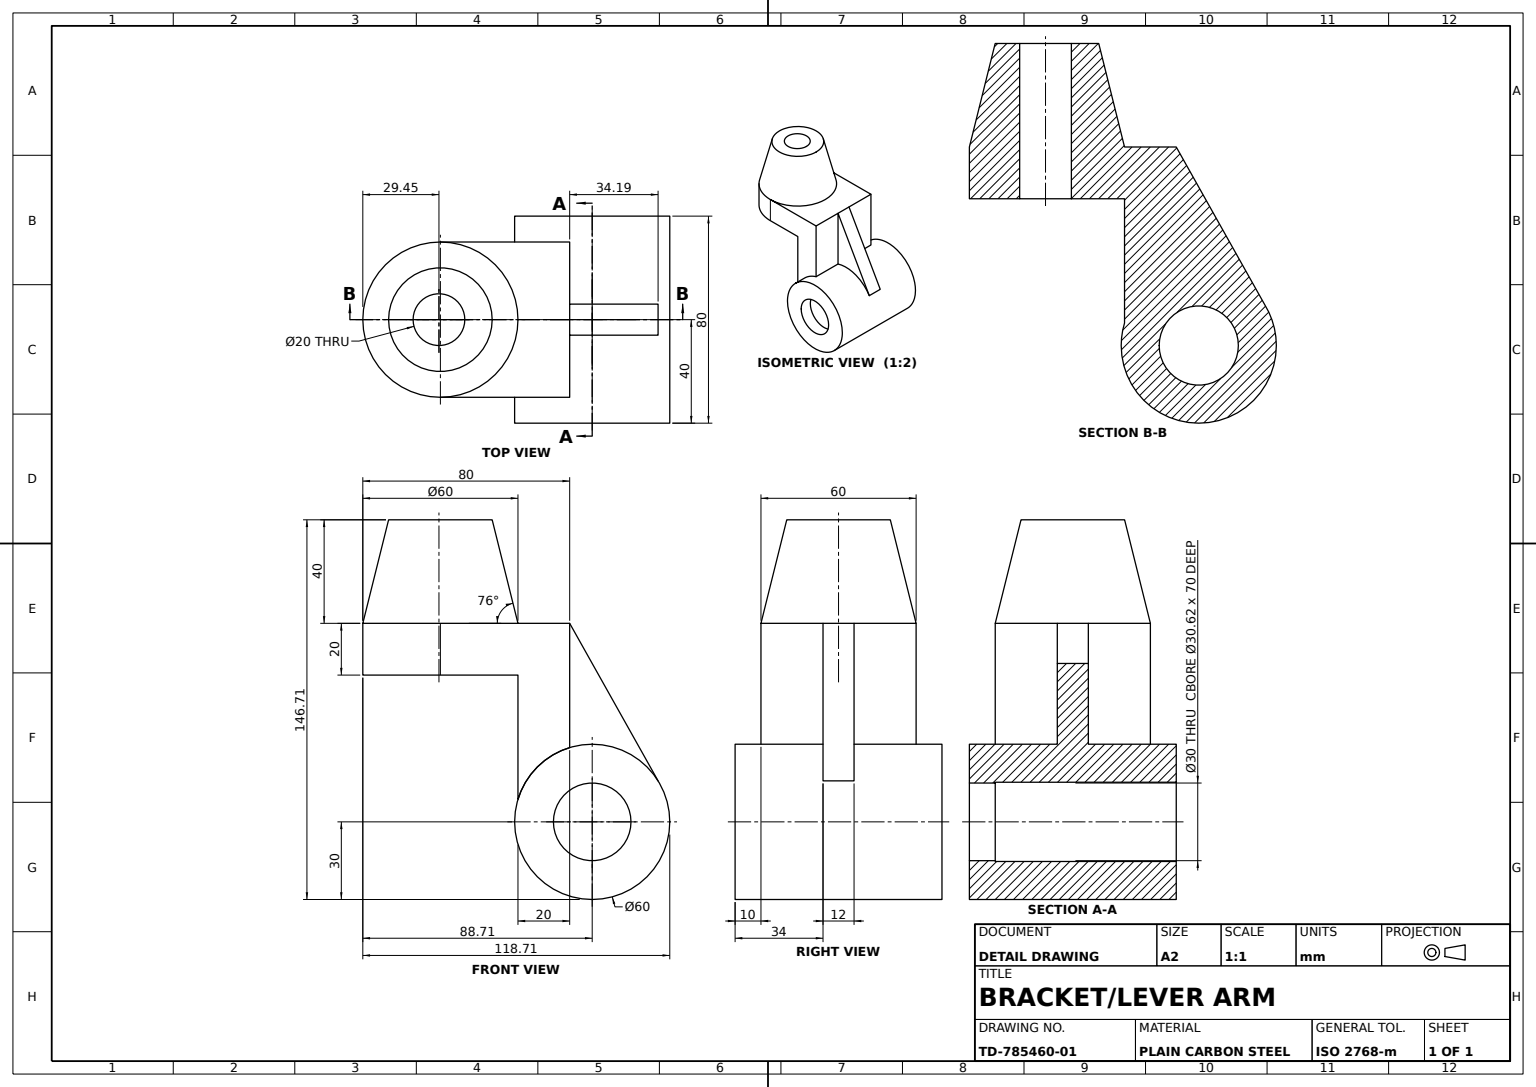
from build123d import *

# Parameters (mm, degrees)
BASE_CYLINDER_SKETCH_R         = 30
BASE_CYLINDER_SKETCH_R_2       = 15
BASE_CYLINDER_60_DEPTH         = 20
SUPPORT_ARM_DEPTH              = 30
HUB_BOSS_A_SKETCH_R            = 30
HUB_BOSS_A_DEPTH               = 10
HUB_BOSS_B_SKETCH_R            = 30
HUB_BOSS_B_DEPTH               = 10
ARM_PAD_SKETCH_R               = 30
ARM_PAD_SKETCH_R_2             = 15
ARM_PAD_DEPTH                  = 10
ARM_BOSS_SKETCH_R              = 30
ARM_BOSS_DEPTH                 = 10
SUPPORT_RIB_12MM_DEPTH         = 6
ARM_POCKET_CUT_DEPTH           = 40
TAPERED_BOSS_SKETCH_R          = 30
TAPERED_BOSS_14DEG_DRAFT_DEPTH = 40
TAPERED_BOSS_14DEG_DRAFT_TAPER = 14
BOSS_HOLE_SKETCH_R             = 10
BOSS_HOLE_20_DEPTH             = 177.046816624
CYLINDER_BORE_SKETCH_R         = 15.308926848
CYLINDER_BORE_DEPTH            = 163.449944447


with BuildPart() as part:
    # Base Cylinder Sketch → Base Cylinder Ø60 (new, symmetric)
    with BuildSketch(Plane.XY):
        Circle(BASE_CYLINDER_SKETCH_R)
        Circle(BASE_CYLINDER_SKETCH_R_2, mode=Mode.SUBTRACT)
    extrude(amount=BASE_CYLINDER_60_DEPTH, both=True)

    # Support Arm Sketch → Support Arm (add, symmetric)
    with BuildSketch(Plane.XY):
        with BuildLine():
            Line((-28.708286934, 56.708286934), (-28.708286934, 8.708286934))
            ThreePointArc((-28.708286934, 8.708286934), (-21.213203436, 21.213203436), (-8.708286934, 28.708286934))
            Line((-8.708286934, 28.708286934), (-8.708286934, 76.708286934))
            Line((-8.708286934, 76.708286934), (-88.708286934, 76.708286934))
            Line((-88.708286934, 76.708286934), (-88.708286934, 56.708286934))
            Line((-88.708286934, 56.708286934), (-28.708286934, 56.708286934))
        make_face()
    extrude(amount=SUPPORT_ARM_DEPTH, both=True)

    # Hub Boss A Sketch → Hub Boss A (add, symmetric)
    with BuildSketch(Plane.XY.offset(20)):
        Circle(HUB_BOSS_A_SKETCH_R)
    extrude(amount=HUB_BOSS_A_DEPTH, both=True)

    # Hub Boss B Sketch → Hub Boss B (add, symmetric)
    with BuildSketch(Plane(origin=(0, 0, -20), x_dir=(-1, 0, 0), z_dir=(0, 0, -1))):
        Circle(HUB_BOSS_B_SKETCH_R)
    extrude(amount=HUB_BOSS_B_DEPTH, both=True)

    # Arm Pad Sketch → Arm Pad (add, symmetric)
    with BuildSketch(Plane.XY.offset(30)):
        with Locations(Location((0, 0, 0), (0, 0, 163.125505702))):
            Circle(ARM_PAD_SKETCH_R)
        Circle(ARM_PAD_SKETCH_R_2, mode=Mode.SUBTRACT)
    extrude(amount=ARM_PAD_DEPTH, both=True)

    # Arm Boss Sketch → Arm Boss (add, symmetric)
    with BuildSketch(Plane(origin=(0, 0, -30), x_dir=(-1, 0, 0), z_dir=(0, 0, -1))):
        Circle(ARM_BOSS_SKETCH_R)
    extrude(amount=ARM_BOSS_DEPTH, both=True)

    # Rib Profile Sketch → Support Rib 12mm (add, symmetric)
    with BuildSketch(Plane.XY):
        with BuildLine():
            Line((-8.708286934, 76.708286934), (-8.708286934, 28.708286934))
            ThreePointArc((-8.708286934, 28.708286934), (10.568877445, 28.076659872), (25.477478309, 15.839763225))
            Line((25.477478309, 15.839763225), (-8.708286934, 76.708286934))
        make_face()
    extrude(amount=SUPPORT_RIB_12MM_DEPTH, both=True)

    # Arm Pocket Sketch → Arm Pocket Cut (cut)
    with BuildSketch(Plane(origin=(0, 76.708286934, 0), x_dir=(1, 0, 0), z_dir=(0, 1, 0))):
        with BuildLine():
            Line((-88.708286934, -30), (-58.708286934, -30))
            ThreePointArc((-58.708286934, -30), (-79.921490343, -21.213203462), (-88.708286934, -7.5e-08))
            Line((-88.708286934, -7.5e-08), (-88.708286934, -30))
        make_face()
        with BuildLine():
            Line((-88.708286934, 30), (-88.708286934, -7.5e-08))
            ThreePointArc((-88.708286934, -7.5e-08), (-79.921490396, 21.213203409), (-58.708286934, 30))
            Line((-58.708286934, 30), (-88.708286934, 30))
        make_face()
    extrude(amount=-ARM_POCKET_CUT_DEPTH, mode=Mode.SUBTRACT)

    # Tapered Boss Sketch → Tapered Boss 14deg Draft (add)
    with BuildSketch(Plane(origin=(0, 76.708286934, 0), x_dir=(1, 0, 0), z_dir=(0, 1, 0))):
        with Locations((-58.708286934, 0)):
            Circle(TAPERED_BOSS_SKETCH_R)
    extrude(amount=TAPERED_BOSS_14DEG_DRAFT_DEPTH, taper=TAPERED_BOSS_14DEG_DRAFT_TAPER)

    # Boss Hole Sketch → Boss Hole Ø20 (cut, through all)
    with BuildSketch(Plane(origin=(0, 116.708286934, 0), x_dir=(1, 0, 0), z_dir=(0, 1, 0))):
        with Locations(Location((-59.262949737, 0, 0), (0, 0, 180))):
            Circle(BOSS_HOLE_SKETCH_R)
    extrude(amount=-BOSS_HOLE_20_DEPTH, mode=Mode.SUBTRACT)

    # Cylinder Bore Sketch → Cylinder Bore (cut, through all)
    with BuildSketch(Plane.XY.offset(30)):
        Circle(CYLINDER_BORE_SKETCH_R)
    extrude(amount=-CYLINDER_BORE_DEPTH, mode=Mode.SUBTRACT)


solid = part.part
